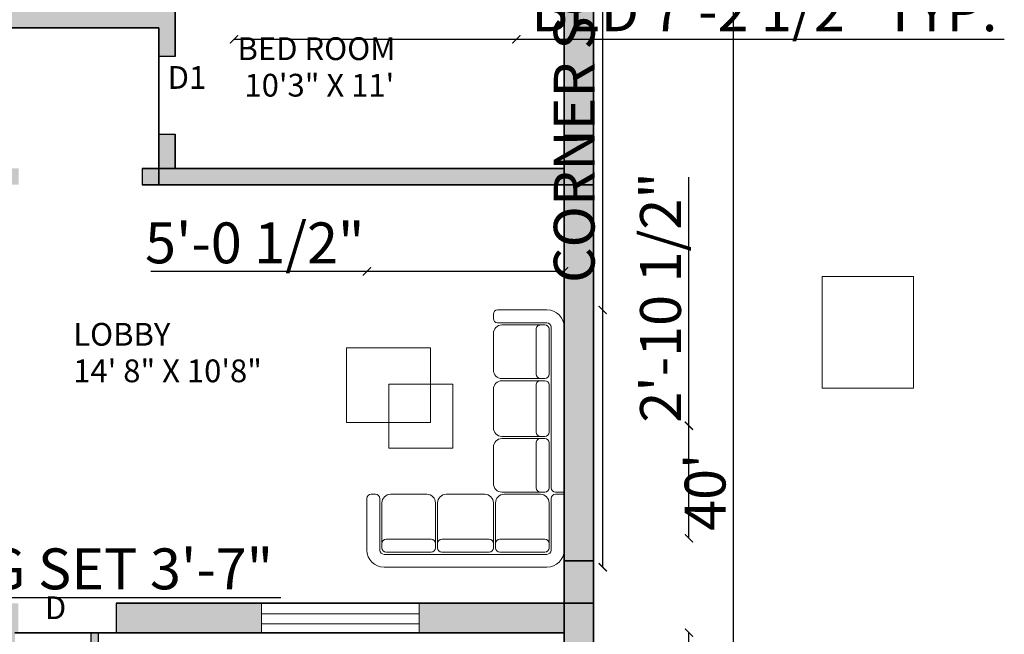
# Model space of a CAD drawing. Units: inches. Extents: x 1858 to 2399, y 1317 to 1943.
# Tile 4 of 8: x 2098 to 2399, y 1554 to 1742. Entities that reach past the tile are written whole.
import ezdxf

# ---------------------------------------------------------------- set-up
doc = ezdxf.new("R2010")
doc.units = ezdxf.units.IN
for name, color, linetype, lineweight in [('A-ANNO-DIMS', 2, 'Continuous', 18), ('A-ANNO-TEXT', 7, 'Continuous', 18), ('A-AREA-IDEN', 7, 'Continuous', 18), ('A-COLS', 7, 'Continuous', 35), ('A-COLS-PATT', 5, 'Continuous', 13), ('A-DOOR', 4, 'Continuous', 25), ('A-FLOR-PATT', 8, 'Continuous', 13), ('A-FURN', 8, 'Continuous', 18), ('A-GENM-REFR', 8, 'Continuous', 13), ('A-WALL', 7, 'Continuous', 35), ('A-WALL-PATT', 1, 'Continuous', 13), ('stairs', 3, 'Continuous', 25), ('window', 4, 'Continuous', 18)]:
    doc.layers.add(name, color=color, linetype=linetype, lineweight=lineweight)
doc.styles.get("Standard").update_dxf_attribs({"font": 'arial.ttf'})
doc.dimstyles.new('ISO-25', dxfattribs={"dimtxt": 12.5, "dimasz": 2.5, "dimexe": 1.25, "dimexo": 0.625, "dimtad": 1, "dimdec": 0, "dimlunit": 4, "dimtxsty": 'Standard', "dimblk": 'ARCHTICK', "dimcen": 2.5, "dimse1": 1, "dimse2": 1, "dimclrd": 3, "dimclrt": 4, "dimadec": 0, "dimazin": 0, "dimtfac": 1, "dimtdec": 0, "dimtmove": 0, "dimatfit": 3, "dimfxl": 1, "dimarcsym": 0})

# ---------------------------------------------------------------- blocks, each defined once
blk = doc.blocks.new('A$C2AFA021D')
for p, q in [((0.8, 2.3), (0.2, 2.3)), ((0.85, 2.2), (0.85, 2.25)), ((0, 2.1), (0, 0.2)), ((0.15, 0.2), (0.15, 2.1)), ((0.175, 1.55), (0.175, 2.075)), ((0.2, 2.15), (0.8, 2.15)), ((0.225, 2.125), (0.275, 2.125)), ((0.75, 2.125), (0.275, 2.125)), ((0.325, 2.075), (0.325, 1.55)), ((0.85, 1.6), (0.85, 2.025)), ((0.275, 1.5), (0.225, 1.5)), ((0.275, 1.5), (0.75, 1.5)), ((0.175, 0.875), (0.175, 1.425)), ((0.225, 1.475), (0.275, 1.475)), ((0.75, 1.475), (0.275, 1.475)), ((0.325, 1.425), (0.325, 0.875)), ((0.85, 0.925), (0.85, 1.375)), ((0.275, 0.825), (0.225, 0.825)), ((0.275, 0.825), (0.75, 0.825)), ((0.975, 0.825), (1.4, 0.825)), ((1.625, 0.825), (2.075, 0.825)), ((2.3, 0.825), (2.725, 0.825)), ((2.9, 0.825), (2.95, 0.825)), ((0.175, 0.225), (0.175, 0.75)), ((0.225, 0.8), (0.275, 0.8)), ((0.75, 0.8), (0.275, 0.8)), ((0.325, 0.75), (0.325, 0.225)), ((0.85, 0.275), (0.85, 0.7)), ((0.875, 0.275), (0.875, 0.725)), ((1.5, 0.725), (1.5, 0.275)), ((1.525, 0.275), (1.525, 0.725)), ((2.175, 0.725), (2.175, 0.275)), ((2.2, 0.275), (2.2, 0.725)), ((2.825, 0.725), (2.825, 0.275)), ((2.85, 0.2), (2.85, 0.775)), ((3, 0.775), (3, 0.2)), ((0.875, 0.275), (0.875, 0.225)), ((1.45, 0.325), (0.925, 0.325)), ((1.5, 0.225), (1.5, 0.275)), ((1.525, 0.275), (1.525, 0.225)), ((2.125, 0.325), (1.575, 0.325)), ((2.175, 0.225), (2.175, 0.275)), ((2.2, 0.275), (2.2, 0.225)), ((2.775, 0.325), (2.25, 0.325)), ((2.825, 0.225), (2.825, 0.275)), ((0.8, 0.15), (0.2, 0.15)), ((0.275, 0.175), (0.225, 0.175)), ((0.275, 0.175), (0.75, 0.175)), ((0.925, 0.175), (1.45, 0.175)), ((0.925, 0.15), (2.8, 0.15)), ((1.575, 0.175), (2.125, 0.175)), ((2.25, 0.175), (2.775, 0.175)), ((0.85, 0), (0.85, 0.1)), ((0.875, 0.1), (0.875, 0)), ((0.2, 0), (0.85, 0)), ((2.8, 0), (0.875, 0))]:
    blk.add_line(p, q)
for centre, radius, start, end in [((0.2, 2.1), 0.2, 90, 180), ((0.8, 2.25), 0.05, 0, 90), ((0.8, 2.2), 0.05, 270, 0), ((0.2, 2.1), 0.05, 90, 180), ((0.225, 2.075), 0.05, 90, 180), ((0.275, 2.075), 0.05, 0, 90), ((0.75, 2.025), 0.1, 0, 90), ((0.225, 1.55), 0.05, 180, 270), ((0.275, 1.55), 0.05, 270, 0), ((0.75, 1.6), 0.1, 270, 0), ((0.225, 1.425), 0.05, 90, 180), ((0.275, 1.425), 0.05, 0, 90), ((0.75, 1.375), 0.1, 360, 90), ((0.75, 0.925), 0.1, 270, 0), ((0.225, 0.875), 0.05, 180, 270), ((0.275, 0.875), 0.05, 270, 0), ((0.975, 0.725), 0.1, 90, 180), ((1.4, 0.725), 0.1, 0, 90), ((1.625, 0.725), 0.1, 90, 180), ((2.075, 0.725), 0.1, 0, 90), ((2.3, 0.725), 0.1, 90, 180), ((2.725, 0.725), 0.1, 0, 90), ((2.9, 0.775), 0.05, 90, 180), ((2.95, 0.775), 0.05, 0, 90), ((0.225, 0.75), 0.05, 90, 180), ((0.275, 0.75), 0.05, 0, 90), ((0.75, 0.7), 0.1, 0, 90), ((0.75, 0.275), 0.1, 270, 0), ((0.925, 0.275), 0.05, 90, 180), ((1.45, 0.275), 0.05, 360, 90), ((1.575, 0.275), 0.05, 90, 180), ((2.125, 0.275), 0.05, 360, 90), ((2.25, 0.275), 0.05, 90, 180), ((2.775, 0.275), 0.05, 360, 90), ((0.2, 0.2), 0.2, 180, 270), ((0.2, 0.2), 0.05, 180, 270), ((0.225, 0.225), 0.05, 180, 270), ((0.275, 0.225), 0.05, 270, 0), ((0.8, 0.1), 0.05, 0, 90), ((0.925, 0.225), 0.05, 180, 270), ((0.925, 0.1), 0.05, 90, 180), ((1.45, 0.225), 0.05, 270, 0), ((1.575, 0.225), 0.05, 180, 270), ((2.125, 0.225), 0.05, 270, 0), ((2.25, 0.225), 0.05, 180, 270), ((2.775, 0.225), 0.05, 270, 0), ((2.8, 0.2), 0.2, 270, 0), ((2.8, 0.2), 0.05, 270, 0)]:
    blk.add_arc(centre, radius, start, end)
blk = doc.blocks.new('_ArchTick')
at = {"color": 0, "linetype": 'ByBlock', "const_width": 0.15}
blk.add_lwpolyline([(-0.5, -0.5), (0.5, 0.5)], dxfattribs=at)
blk = doc.blocks.new('*D13')
at = {"layer": 'A-ANNO-DIMS', "color": 0, "lineweight": -2, "transparency": 16777216}
blk.add_line((2316.13, 1837.34), (2316.13, 1357.34), dxfattribs=at)
at = {"layer": 'Defpoints', "color": 0, "transparency": 16777216}
for p in [(2273.38, 1837.34), (2273.38, 1357.34), (2316.13, 1357.34)]:
    blk.add_point(p, dxfattribs=at)
at = {"layer": 'A-ANNO-DIMS', "color": 0, "lineweight": -2, "transparency": 16777216, "xscale": 2.5, "yscale": 2.5, "zscale": 2.5}
for p, rotation in [((2316.13, 1837.34), 90), ((2316.13, 1357.34), 270)]:
    blk.add_blockref('_ArchTick', p, dxfattribs=dict(at, rotation=rotation))
at = {"layer": 'A-ANNO-DIMS', "color": 0, "transparency": 16777216, "insert": (2309.12, 1597.34), "char_height": 12.5, "attachment_point": 5, "rotation": 90}
blk.add_mtext("40'", dxfattribs=at)
blk = doc.blocks.new('*D15')
at = {"layer": 'A-ANNO-DIMS', "color": 3, "lineweight": -2, "transparency": 16777216}
for p, q in [((2163.42, 1735.85), (2249.76, 1735.85)), ((2249.76, 1735.85), (2399.03, 1735.85))]:
    blk.add_line(p, q, dxfattribs=at)
at = {"layer": 'Defpoints', "color": 0, "transparency": 16777216}
for p in [(2163.42, 1748.8), (2249.76, 1748.8), (2249.76, 1735.85)]:
    blk.add_point(p, dxfattribs=at)
at = {"layer": 'A-ANNO-DIMS', "color": 3, "lineweight": -2, "transparency": 16777216, "xscale": 2.5, "yscale": 2.5, "zscale": 2.5, "rotation": 180}
blk.add_blockref('_ArchTick', (2163.42, 1735.85), dxfattribs=at)
at = {"layer": 'A-ANNO-DIMS', "color": 3, "lineweight": -2, "transparency": 16777216, "xscale": 2.5, "yscale": 2.5, "zscale": 2.5}
blk.add_blockref('_ArchTick', (2249.76, 1735.85), dxfattribs=at)
at = {"layer": 'A-ANNO-DIMS', "color": 4, "transparency": 16777216, "insert": (2325.64, 1742.94), "char_height": 12.5, "attachment_point": 5}
blk.add_mtext('BED 7\'-2 1/2" TYP.', dxfattribs=at)
blk = doc.blocks.new('*D17')
at = {"layer": 'A-ANNO-DIMS', "color": 3, "lineweight": -2, "transparency": 16777216}
for p, q in [((2276.18, 1653.07), (2276.18, 1851.95)), ((2276.18, 1574.39), (2276.18, 1653.07))]:
    blk.add_line(p, q, dxfattribs=at)
at = {"layer": 'Defpoints', "color": 0, "transparency": 16777216}
for p in [(2264.38, 1653.07), (2276.18, 1653.07), (2264.38, 1574.39)]:
    blk.add_point(p, dxfattribs=at)
at = {"layer": 'A-ANNO-DIMS', "color": 3, "lineweight": -2, "transparency": 16777216, "xscale": 2.5, "yscale": 2.5, "zscale": 2.5}
for p, rotation in [((2276.18, 1653.07), 90), ((2276.18, 1574.39), 270)]:
    blk.add_blockref('_ArchTick', p, dxfattribs=dict(at, rotation=rotation))
at = {"layer": 'A-ANNO-DIMS', "color": 4, "transparency": 16777216, "insert": (2269.09, 1753.76), "char_height": 12.5, "attachment_point": 5, "rotation": 90}
blk.add_mtext('CORNER SOFA 6\'-6 1/2"', dxfattribs=at)
blk = doc.blocks.new('*D18')
at = {"layer": 'A-ANNO-DIMS', "color": 3, "lineweight": -2, "transparency": 16777216}
for p, q in [((2204.05, 1664.87), (2137.95, 1664.87)), ((2264.38, 1664.87), (2204.05, 1664.87))]:
    blk.add_line(p, q, dxfattribs=at)
at = {"layer": 'Defpoints', "color": 0, "transparency": 16777216}
for p in [(2204.05, 1664.87), (2204.05, 1653.07), (2264.38, 1653.07)]:
    blk.add_point(p, dxfattribs=at)
at = {"layer": 'A-ANNO-DIMS', "color": 3, "lineweight": -2, "transparency": 16777216, "xscale": 2.5, "yscale": 2.5, "zscale": 2.5, "rotation": 180}
blk.add_blockref('_ArchTick', (2204.05, 1664.87), dxfattribs=at)
at = {"layer": 'A-ANNO-DIMS', "color": 3, "lineweight": -2, "transparency": 16777216, "xscale": 2.5, "yscale": 2.5, "zscale": 2.5}
blk.add_blockref('_ArchTick', (2264.38, 1664.87), dxfattribs=at)
at = {"layer": 'A-ANNO-DIMS', "color": 4, "transparency": 16777216, "insert": (2169.75, 1671.96), "char_height": 12.5, "attachment_point": 5}
blk.add_mtext('5\'-0 1/2"', dxfattribs=at)
blk = doc.blocks.new('*D25')
at = {"layer": 'A-ANNO-DIMS', "color": 3, "lineweight": -2, "transparency": 16777216}
for p, q in [((1993.57, 1565.17), (2036.62, 1565.17)), ((2036.62, 1565.17), (2177.76, 1565.17))]:
    blk.add_line(p, q, dxfattribs=at)
at = {"layer": 'Defpoints', "color": 0, "transparency": 16777216}
for p in [(1993.57, 1571.63), (2036.62, 1571.63), (2036.62, 1565.17)]:
    blk.add_point(p, dxfattribs=at)
at = {"layer": 'A-ANNO-DIMS', "color": 3, "lineweight": -2, "transparency": 16777216, "xscale": 2.5, "yscale": 2.5, "zscale": 2.5, "rotation": 180}
blk.add_blockref('_ArchTick', (1993.57, 1565.17), dxfattribs=at)
at = {"layer": 'A-ANNO-DIMS', "color": 3, "lineweight": -2, "transparency": 16777216, "xscale": 2.5, "yscale": 2.5, "zscale": 2.5}
blk.add_blockref('_ArchTick', (2036.62, 1565.17), dxfattribs=at)
at = {"layer": 'A-ANNO-DIMS', "color": 4, "transparency": 16777216, "insert": (2108.44, 1572.26), "char_height": 12.5, "attachment_point": 5}
blk.add_mtext('DINING SET 3\'-7"', dxfattribs=at)
blk = doc.blocks.new('*D29')
at = {"layer": 'A-ANNO-DIMS', "color": 3, "lineweight": -2, "transparency": 16777216}
blk.add_line((2302.58, 1366.34), (2302.58, 1554.34), dxfattribs=at)
at = {"layer": 'Defpoints', "color": 0, "transparency": 16777216}
for p in [(2264.38, 1554.34), (2302.58, 1554.34), (2264.38, 1366.34)]:
    blk.add_point(p, dxfattribs=at)
at = {"layer": 'A-ANNO-DIMS', "color": 3, "lineweight": -2, "transparency": 16777216, "xscale": 2.5, "yscale": 2.5, "zscale": 2.5}
for p, rotation in [((2302.58, 1554.34), 90), ((2302.58, 1366.34), 270)]:
    blk.add_blockref('_ArchTick', p, dxfattribs=dict(at, rotation=rotation))
at = {"layer": 'A-ANNO-DIMS', "color": 4, "transparency": 16777216, "insert": (2295.57, 1460.34), "char_height": 12.5, "attachment_point": 5, "rotation": 90}
blk.add_mtext('15\'-8"', dxfattribs=at)
blk = doc.blocks.new('*D50')
at = {"layer": 'A-ANNO-DIMS', "color": 3, "lineweight": -2, "transparency": 16777216}
for p, q in [((2097.46, 1917.54), (2127.41, 1917.54)), ((2127.41, 1917.54), (2164.6, 1917.54))]:
    blk.add_line(p, q, dxfattribs=at)
at = {"layer": 'Defpoints', "color": 0, "transparency": 16777216}
for p in [(2127.41, 1917.54), (2097.46, 1563.34), (2127.41, 1563.34)]:
    blk.add_point(p, dxfattribs=at)
at = {"layer": 'A-ANNO-DIMS', "color": 3, "lineweight": -2, "transparency": 16777216, "xscale": 2.5, "yscale": 2.5, "zscale": 2.5, "rotation": 180}
blk.add_blockref('_ArchTick', (2097.46, 1917.54), dxfattribs=at)
at = {"layer": 'A-ANNO-DIMS', "color": 3, "lineweight": -2, "transparency": 16777216, "xscale": 2.5, "yscale": 2.5, "zscale": 2.5}
blk.add_blockref('_ArchTick', (2127.41, 1917.54), dxfattribs=at)
at = {"layer": 'A-ANNO-DIMS', "color": 4, "transparency": 16777216, "insert": (2147.25, 1924.55), "char_height": 12.5, "attachment_point": 5}
blk.add_mtext('2\'-6"', dxfattribs=at)
blk = doc.blocks.new('*D51')
at = {"layer": 'A-ANNO-DIMS', "color": 3, "lineweight": -2, "transparency": 16777216}
for p, q in [((2127.41, 1917.54), (2171.86, 1917.54)), ((2171.86, 1917.54), (2237.95, 1917.54))]:
    blk.add_line(p, q, dxfattribs=at)
at = {"layer": 'Defpoints', "color": 0, "transparency": 16777216}
for p in [(2171.86, 1917.54), (2127.41, 1563.34), (2171.86, 1563.34)]:
    blk.add_point(p, dxfattribs=at)
at = {"layer": 'A-ANNO-DIMS', "color": 3, "lineweight": -2, "transparency": 16777216, "xscale": 2.5, "yscale": 2.5, "zscale": 2.5, "rotation": 180}
blk.add_blockref('_ArchTick', (2127.41, 1917.54), dxfattribs=at)
at = {"layer": 'A-ANNO-DIMS', "color": 3, "lineweight": -2, "transparency": 16777216, "xscale": 2.5, "yscale": 2.5, "zscale": 2.5}
blk.add_blockref('_ArchTick', (2171.86, 1917.54), dxfattribs=at)
at = {"layer": 'A-ANNO-DIMS', "color": 4, "transparency": 16777216, "insert": (2206.15, 1924.63), "char_height": 12.5, "attachment_point": 5}
blk.add_mtext('3\'-8 1/2"', dxfattribs=at)
blk = doc.blocks.new('*D52')
at = {"layer": 'A-ANNO-DIMS', "color": 3, "lineweight": -2, "transparency": 16777216}
blk.add_line((2171.86, 1917.54), (2220, 1917.54), dxfattribs=at)
at = {"layer": 'Defpoints', "color": 0, "transparency": 16777216}
for p in [(2220, 1917.54), (2171.86, 1563.34), (2220, 1563.34)]:
    blk.add_point(p, dxfattribs=at)
at = {"layer": 'A-ANNO-DIMS', "color": 3, "lineweight": -2, "transparency": 16777216, "xscale": 2.5, "yscale": 2.5, "zscale": 2.5, "rotation": 180}
blk.add_blockref('_ArchTick', (2171.86, 1917.54), dxfattribs=at)
at = {"layer": 'A-ANNO-DIMS', "color": 3, "lineweight": -2, "transparency": 16777216, "xscale": 2.5, "yscale": 2.5, "zscale": 2.5}
blk.add_blockref('_ArchTick', (2220, 1917.54), dxfattribs=at)
at = {"layer": 'A-ANNO-DIMS', "color": 4, "transparency": 16777216, "insert": (2195.93, 1924.55), "char_height": 12.5, "attachment_point": 5}
blk.add_mtext('4\'-0"', dxfattribs=at)
blk = doc.blocks.new('*D58')
at = {"layer": 'A-ANNO-DIMS', "color": 3, "lineweight": -2, "transparency": 16777216}
for p, q in [((1884.18, 1730.57), (1884.18, 1767.76)), ((1884.18, 1706.78), (1884.18, 1730.57))]:
    blk.add_line(p, q, dxfattribs=at)
at = {"layer": 'Defpoints', "color": 0, "transparency": 16777216}
for p in [(1884.18, 1730.57), (2145.38, 1730.57), (2145.38, 1706.78)]:
    blk.add_point(p, dxfattribs=at)
at = {"layer": 'A-ANNO-DIMS', "color": 3, "lineweight": -2, "transparency": 16777216, "xscale": 2.5, "yscale": 2.5, "zscale": 2.5}
for p, rotation in [((1884.18, 1730.57), 90), ((1884.18, 1706.78), 270)]:
    blk.add_blockref('_ArchTick', p, dxfattribs=dict(at, rotation=rotation))
at = {"layer": 'A-ANNO-DIMS', "color": 4, "transparency": 16777216, "insert": (1877.17, 1750.41), "char_height": 12.5, "attachment_point": 5, "rotation": 90}
blk.add_mtext('2\'-0"', dxfattribs=at)
blk = doc.blocks.new('*D59')
at = {"layer": 'A-ANNO-DIMS', "color": 3, "lineweight": -2, "transparency": 16777216}
for p, q in [((2302.58, 1617.63), (2302.58, 1693.66)), ((2302.58, 1583.24), (2302.58, 1617.63))]:
    blk.add_line(p, q, dxfattribs=at)
at = {"layer": 'Defpoints', "color": 0, "transparency": 16777216}
for p in [(2092.38, 1617.63), (2302.58, 1617.63), (2092.38, 1583.24)]:
    blk.add_point(p, dxfattribs=at)
at = {"layer": 'A-ANNO-DIMS', "color": 3, "lineweight": -2, "transparency": 16777216, "xscale": 2.5, "yscale": 2.5, "zscale": 2.5}
for p, rotation in [((2302.58, 1617.63), 90), ((2302.58, 1583.24), 270)]:
    blk.add_blockref('_ArchTick', p, dxfattribs=dict(at, rotation=rotation))
at = {"layer": 'A-ANNO-DIMS', "color": 4, "transparency": 16777216, "insert": (2295.49, 1656.89), "char_height": 12.5, "attachment_point": 5, "rotation": 90}
blk.add_mtext('2\'-10 1/2"', dxfattribs=at)

msp = doc.modelspace()

# ---------------------------------------------------------------- hatches: boundary and pattern name
at = {"layer": 'A-COLS-PATT'}
h = msp.add_hatch(color=256, dxfattribs=at)
h.dxf.hatch_style = 1
h.paths.add_polyline_path([(2273.38, 1706.46), (2264.38, 1706.46), (2264.38, 1691.34), (2273.38, 1691.34)])
h.paths.add_polyline_path([(2273.38, 1576.35), (2264.38, 1576.35), (2264.38, 1563.34), (2273.38, 1563.34)])
h.paths.add_polyline_path([(2241.64, 1366.34), (2228.69, 1366.34), (2228.69, 1357.34), (2241.64, 1357.34)])
h.paths.add_polyline_path([(2096.38, 1366.34), (2085.57, 1366.34), (2085.57, 1357.34), (2096.38, 1357.34)])
h.paths.add_polyline_path([(1963.94, 1366.34), (1951.36, 1366.34), (1951.36, 1357.34), (1963.94, 1357.34)])
h = msp.add_hatch(color=256, dxfattribs=at)
h.dxf.hatch_style = 1
h.paths.add_polyline_path([(2092.38, 1705.02), (2087.38, 1705.02), (2087.38, 1696.34), (2092.38, 1696.34)])
h.paths.add_polyline_path([(2097.51, 1696.34), (2092.38, 1696.34), (2092.38, 1691.34), (2097.51, 1691.34)])
h.paths.add_polyline_path([(2140.38, 1696.34), (2135.36, 1696.34), (2135.36, 1691.34), (2140.38, 1691.34)])
h.paths.add_polyline_path([(2145.38, 1706.78), (2140.38, 1706.78), (2140.38, 1696.34), (2145.38, 1696.34)])
h.paths.add_polyline_path([(2097.46, 1563.34), (2092.38, 1563.34), (2087.38, 1563.34), (2087.38, 1554.34), (2096.38, 1554.34), (2097.46, 1554.34)])
at = {"layer": 'A-FLOR-PATT'}
h = msp.add_hatch(dxfattribs=at)
h.set_pattern_fill('ANGLE', color=256)
h.set_pattern_definition([(0, (0, 0), (0, 6.985), [5.08, -1.905]), (90, (0, 0), (-6.985, 4e-16), [5.08, -1.905])])
h.paths.add_polyline_path([(2058.38, 1691.34), (2005.38, 1691.34), (2005.38, 1696.34), (1977.99, 1696.34), (1977.99, 1691.34), (1967.38, 1691.34), (1967.38, 1643.34), (2026.65, 1643.34), (2026.65, 1651.34), (2033.15, 1651.34), (2031.15, 1657.34, -0.501323), (2036.1, 1676.2, -0.132891), (2038.19, 1676.2, -0.501317), (2043.15, 1657.34), (2041.15, 1651.34), (2044.15, 1651.34), (2044.15, 1652.84), (2047.15, 1652.84), (2047.15, 1651.34), (2047.65, 1651.34), (2047.65, 1643.34), (2058.38, 1643.34)])
h.paths.add_polyline_path([(2140.38, 1828.34), (2130, 1828.34), (2130, 1820.34), (2123.5, 1820.34), (2125.5, 1814.34, -0.501323), (2120.55, 1795.48, -0.132891), (2118.46, 1795.48, -0.501317), (2113.5, 1814.34), (2115.5, 1820.34), (2112.5, 1820.34), (2112.5, 1818.84), (2109.5, 1818.84), (2109.5, 1820.34), (2109, 1820.34), (2109, 1828.34), (2107.67, 1828.34), (2092.38, 1828.34), (2092.38, 1744.34), (2140.38, 1744.34)])
h.paths.add_polyline_path([(1981.03, 1683.02), (1996.96, 1683.02), (1996.96, 1693.5), (1981.03, 1693.5)], flags=24)
h.paths.add_polyline_path([(1975.79, 1660.59), (2014.55, 1660.59), (2014.55, 1671.04), (1975.79, 1671.04)], flags=24)
h.paths.add_polyline_path([(1975.73, 1671.6), (2013.37, 1671.6), (2013.37, 1682.41), (1975.73, 1682.41)], flags=24)
h.paths.add_polyline_path([(2096.15, 1778.17), (2126.05, 1778.17), (2126.05, 1788.61), (2096.15, 1788.61)], flags=24)
h.paths.add_polyline_path([(2096.09, 1789.17), (2133.73, 1789.17), (2133.73, 1799.98), (2096.09, 1799.98)], flags=24)
at = {"layer": 'A-WALL-PATT'}
h = msp.add_hatch(color=256, dxfattribs=at)
h.dxf.hatch_style = 1
h.paths.add_polyline_path([(1967.38, 1742.58), (1958.38, 1742.58), (1958.38, 1700.89), (1967.38, 1700.89)])
h.paths.add_polyline_path([(1967.38, 1685.05), (1958.38, 1685.05), (1958.38, 1672.42), (1967.38, 1672.42)], flags=17)
h.paths.add_polyline_path([(2092.38, 1643.34), (2087.38, 1643.34), (2063.38, 1643.34), (2063.38, 1691.34), (2087.38, 1691.34), (2092.38, 1691.34), (2092.38, 1696.34), (2087.38, 1696.34), (2005.38, 1696.34), (2005.38, 1691.34), (2058.38, 1691.34), (2058.38, 1643.34), (1967.38, 1643.34), (1967.38, 1652.51), (1958.38, 1652.51), (1958.38, 1625.4), (1967.38, 1625.4), (1967.38, 1638.34), (2087.38, 1638.34), (2087.38, 1617.63), (2092.38, 1617.63)])
h.paths.add_polyline_path([(1967.38, 1591.74), (1958.38, 1591.74), (1958.38, 1571.83), (1967.38, 1571.83)])
h.paths.add_polyline_path([(1967.38, 1554.34), (2002.1, 1554.34), (2002.1, 1559.34), (1967.38, 1559.34), (1958.38, 1559.34), (1958.38, 1536.07), (1967.38, 1536.07)])
h.paths.add_polyline_path([(2087.38, 1559.34), (2042.3, 1559.34), (2042.3, 1554.34), (2087.38, 1554.34)])
h.paths.add_polyline_path([(2092.38, 1583.24), (2087.38, 1583.24), (2087.38, 1563.34), (2092.38, 1563.34)])
h.paths.add_polyline_path([(2096.38, 1554.34), (2087.38, 1554.34), (2087.38, 1481.51), (2096.38, 1473.96)])
h.paths.add_polyline_path([(2084.48, 1476.34), (2050.44, 1476.34), (2050.44, 1467.34), (2089.85, 1467.34)])
h.paths.add_polyline_path([(2002.33, 1476.34), (1977.97, 1476.34), (1967.38, 1467.34), (2002.33, 1467.34)])
h.paths.add_polyline_path([(1967.38, 1488.33), (1958.38, 1488.33), (1958.38, 1474.25), (1967.38, 1482.01)])
h.paths.add_polyline_path([(2121.99, 1554.34), (2119.71, 1554.34), (2119.71, 1532.61), (2096.38, 1532.61), (2096.38, 1529.65), (2121.99, 1529.65)])
h.paths.add_polyline_path([(2171.86, 1563.34), (2127.41, 1563.34), (2127.41, 1554.34), (2171.86, 1554.34)])
h.paths.add_polyline_path([(2264.38, 1563.34), (2220, 1563.34), (2220, 1554.34), (2264.38, 1554.34)])
h.paths.add_polyline_path([(2273.38, 1563.34), (2264.38, 1563.34), (2264.38, 1366.34), (2241.64, 1366.34), (2241.64, 1357.34), (2273.38, 1357.34)])
h.paths.add_polyline_path([(2273.38, 1691.34), (2264.38, 1691.34), (2264.38, 1576.35), (2273.38, 1576.35)])
h.paths.add_polyline_path([(2273.38, 1827.14), (2264.38, 1823.36), (2264.38, 1706.46), (2273.38, 1706.46)])
h.paths.add_polyline_path([(2265.79, 1837.34), (2234.56, 1837.34), (2234.56, 1828.34), (2258.24, 1828.34)])
h.paths.add_polyline_path([(2186.7, 1837.34), (2131.33, 1837.34), (2131.33, 1828.34), (2186.7, 1828.34)])
h.paths.add_polyline_path([(2107.67, 1837.34), (2097.64, 1837.34), (2097.64, 1828.34), (2107.67, 1828.34)])
h.paths.add_polyline_path([(2082.58, 1837.34), (2051.43, 1837.34), (2051.43, 1828.34), (2082.58, 1828.34)])
h.paths.add_polyline_path([(2092.38, 1828.34), (2087.38, 1828.34), (2087.38, 1729.93), (2092.38, 1729.93), (2092.38, 1739.34), (2140.38, 1739.34), (2140.38, 1730.57), (2145.38, 1730.57), (2145.38, 1828.34), (2140.38, 1828.34), (2140.38, 1744.34), (2092.38, 1744.34)])
h.paths.add_polyline_path([(1989.86, 1837.34), (1977.66, 1837.34), (1977.66, 1828.34), (1989.86, 1828.34)])
h.paths.add_polyline_path([(1922.38, 1822.27), (1913.38, 1826.41), (1913.38, 1357.34), (1951.36, 1357.34), (1951.36, 1366.34), (1922.38, 1366.34)])
h.paths.add_polyline_path([(1967.38, 1828.34), (1958.38, 1828.34), (1958.38, 1791.57), (1967.38, 1791.57)])
h = msp.add_hatch(color=256, dxfattribs=at)
h.dxf.hatch_style = 1
h.paths.add_polyline_path([(2264.38, 1696.34), (2145.38, 1696.34), (2140.38, 1696.34), (2140.38, 1691.34), (2264.38, 1691.34)])

# ---------------------------------------------------------------- linework, layer by layer
at = {"layer": 'A-COLS'}
for p, q in [((2264.38, 1706.46), (2273.38, 1706.46)), ((2145.38, 1696.34), (2140.38, 1696.34)), ((2140.38, 1696.34), (2140.38, 1691.34)), ((2264.38, 1691.34), (2273.38, 1691.34)), ((2264.38, 1576.35), (2273.38, 1576.35)), ((2264.38, 1563.34), (2273.38, 1563.34))]:
    msp.add_line(p, q, dxfattribs=at)
at = {"layer": 'A-DOOR'}
for p, q in [((2145.38, 1730.57), (2140.38, 1730.57)), ((2140.38, 1706.78), (2145.38, 1706.78)), ((2135.36, 1696.34), (2135.36, 1691.34)), ((2127.41, 1563.34), (2127.41, 1554.34))]:
    msp.add_line(p, q, dxfattribs=at)
at = {"layer": 'A-FURN'}
for points in [[(2197.84, 1641.43), (2223.5, 1641.43), (2223.5, 1618.63), (2197.84, 1618.63)], [(2210.76, 1630.41), (2230.34, 1630.41), (2230.34, 1610.84), (2210.76, 1610.84)]]:
    msp.add_lwpolyline(points, close=True, dxfattribs=at)
at = {"layer": 'A-GENM-REFR'}
msp.add_lwpolyline([(2343.27, 1663.28), (2371.27, 1663.28), (2371.27, 1629.17), (2343.27, 1629.17)], close=True, dxfattribs=at)
at = {"layer": 'A-WALL'}
for p, q in [((2145.38, 1730.57), (2145.38, 1828.34)), ((2264.38, 1828.34), (2264.38, 1366.34)), ((2092.38, 1739.34), (2140.38, 1739.34)), ((2140.38, 1696.34), (2140.38, 1739.34)), ((2145.38, 1696.34), (2145.38, 1706.78)), ((2135.36, 1696.34), (2140.38, 1696.34)), ((2145.38, 1696.34), (2264.38, 1696.34)), ((2135.36, 1691.34), (2264.38, 1691.34)), ((2127.41, 1563.34), (2264.38, 1563.34)), ((2096.38, 1554.34), (2264.38, 1554.34))]:
    msp.add_line(p, q, dxfattribs=at)
msp.add_lwpolyline([(1949.42, 1837.34), (2273.38, 1837.34), (2273.38, 1357.34), (1913.38, 1357.34), (1913.38, 1826.41)], dxfattribs=at)
at = {"layer": 'stairs'}
for p, q in [((2119.71, 1532.61), (2119.71, 1554.34)), ((2121.99, 1529.65), (2121.99, 1554.34))]:
    msp.add_line(p, q, dxfattribs=at)
at = {"layer": 'window'}
for p, q in [((2171.86, 1563.34), (2171.86, 1554.34)), ((2220, 1563.34), (2171.86, 1563.34)), ((2220, 1554.34), (2220, 1563.34)), ((2171.86, 1560.14), (2220, 1560.14)), ((2171.86, 1557.05), (2220, 1557.05)), ((2171.86, 1554.34), (2220, 1554.34))]:
    msp.add_line(p, q, dxfattribs=at)

# ---------------------------------------------------------------- block references
at = {"layer": 'A-FURN', "xscale": 26.2273040101081, "yscale": 26.2273040101081, "zscale": 26.2273040101081, "rotation": 90}
msp.add_blockref('A$C2AFA021D', (2264.38, 1574.39), dxfattribs=at)

# ---------------------------------------------------------------- texts
at = {"layer": 'A-ANNO-TEXT'}
for s, p in [('D1', (2143.12, 1720.69)), ('D', (2105.55, 1558.5))]:
    msp.add_text(s, height=6.96, dxfattribs=at).set_placement(p)
at = {"layer": 'A-AREA-IDEN'}
for s, height, p in [('BED ROOM', 6.96, (2164.47, 1729.5)), (' 10\'3" X 11\'', 6.9604, (2164.47, 1718.32)), ('LOBBY', 6.96, (2114.23, 1642.14)), ('14\' 8" X 10\'8"', 6.9604, (2114.23, 1630.96))]:
    msp.add_text(s, height=height, dxfattribs=at).set_placement(p)

# ---------------------------------------------------------------- dimensions: what is measured, and where the dimension line sits
at = {"layer": 'A-ANNO-DIMS'}
for base, p1, p2, picture, middle in [((2171.8564, 1917.5395), (2127.4089, 1563.3395), (2171.8564, 1563.3395), '*D51', (2206.1547, 1924.6319)), ((2127.4089, 1917.5395), (2097.4626, 1563.3395), (2127.4089, 1563.3395), '*D50', (2147.2545, 1924.5467)), ((2220, 1917.54), (2171.86, 1563.34), (2220, 1563.34), '*D52', (2195.93, 1924.55))]:
    dim = msp.add_linear_dim(base=base, p1=p1, p2=p2, dimstyle='ISO-25', override={"dimdec": 1, "dimlfac": 1, "dimrnd": 0, "dimzin": 1, "dimdsep": 46, "dimlunit": 4, "dimfrac": 2}, dxfattribs=at)
    dim.commit()
    dim.dimension.update_dxf_attribs({"geometry": picture, "text_midpoint": middle})
dim = msp.add_linear_dim(base=(2276.18, 1653.07), p1=(2264.38, 1574.39), p2=(2264.38, 1653.07), angle=90, text='CORNER SOFA <>', dimstyle='ISO-25', override={"dimdec": 1, "dimlfac": 1, "dimrnd": 0, "dimzin": 1, "dimdsep": 46, "dimlunit": 4, "dimfrac": 2}, dxfattribs=at)
dim.commit()
dim.dimension.update_dxf_attribs({"geometry": '*D17', "text_midpoint": (2269.09, 1753.76)})
for base, p1, p2, angle, override, picture, middle in [((2316.13, 1357.34), (2273.38, 1837.34), (2273.38, 1357.34), 90, {"dimclrd": 0, "dimclre": 0, "dimclrt": 0}, '*D13', (2309.12, 1597.34)), ((1884.18, 1730.57), (2145.38, 1706.78), (2145.38, 1730.57), 90, {"dimdec": 1, "dimlfac": 1, "dimrnd": 0, "dimzin": 1, "dimdsep": 46, "dimlunit": 4, "dimfrac": 2}, '*D58', (1877.17, 1750.41)), ((2302.58, 1617.63), (2092.38, 1583.24), (2092.38, 1617.63), 90, {"dimdec": 1, "dimlfac": 1, "dimrnd": 0, "dimzin": 1, "dimdsep": 46, "dimlunit": 4, "dimfrac": 2}, '*D59', (2295.49, 1656.89)), ((2204.05, 1664.87), (2264.38, 1653.07), (2204.05, 1653.07), 180, {"dimdec": 1, "dimlfac": 1, "dimrnd": 0, "dimzin": 1, "dimdsep": 46, "dimlunit": 4, "dimfrac": 2}, '*D18', (2169.75, 1671.96)), ((2302.58, 1554.34), (2264.38, 1366.34), (2264.38, 1554.34), 90, {"dimdec": 1, "dimlfac": 1, "dimrnd": 0, "dimzin": 1, "dimdsep": 46, "dimlunit": 4, "dimfrac": 2}, '*D29', (2295.57, 1460.34))]:
    dim = msp.add_linear_dim(base=base, p1=p1, p2=p2, angle=angle, dimstyle='ISO-25', override=override, dxfattribs=at)
    dim.commit()
    dim.dimension.update_dxf_attribs({"geometry": picture, "text_midpoint": middle})
for base, p1, p2, text, picture, middle in [((2249.76, 1735.85), (2163.42, 1748.8), (2249.76, 1748.8), 'BED <> TYP.', '*D15', (2325.64, 1742.94)), ((2036.6194, 1565.1722), (1993.5737, 1571.629), (2036.6194, 1571.629), 'DINING SET <>', '*D25', (2108.439, 1572.2646))]:
    dim = msp.add_linear_dim(base=base, p1=p1, p2=p2, text=text, dimstyle='ISO-25', override={"dimdec": 1, "dimlfac": 1, "dimrnd": 0, "dimzin": 1, "dimdsep": 46, "dimlunit": 4, "dimfrac": 2}, dxfattribs=at)
    dim.commit()
    dim.dimension.update_dxf_attribs({"geometry": picture, "text_midpoint": middle})

doc.saveas('drawing.dxf')
